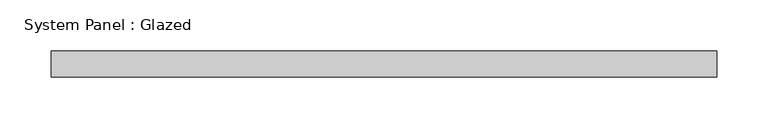
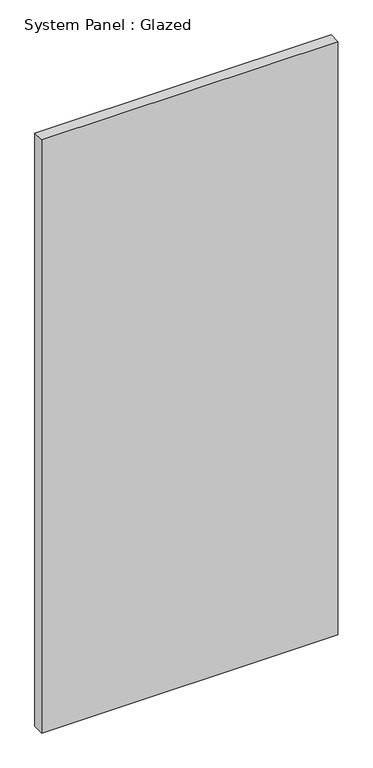
"""IFC4 building model written with IfcOpenShell, lengths in millimetres: plate geometry, System Panel : Glazed."""

from ifc_helpers import new_model, si_unit, origin, origin_with_axes, place, context, project, spatial, polyline, outline, extrude, source, transform, mapped, element, save


def system_panel_glazed_27f6d1d6(model_context):
    return source(origin(), model_context, "Body", "SweptSolid", [
        extrude(outline(polyline([(323.85, 19.05), (-323.85, 19.05), (-323.85, 44.45), (323.85, 44.45), (323.85, 19.05)])), origin_with_axes(), (0.0, 0.0, 1.0), 1371.695751),
    ])


if __name__ == "__main__":
    model = new_model("IFC4")
    model_context = context("Model", 3, world=origin())
    ifc_project = project(units=[si_unit("LENGTHUNIT", "METRE", prefix="MILLI")], contexts=[model_context])
    site = spatial("IfcSite", under=ifc_project)
    building = spatial("IfcBuilding", under=site)
    placement = place(None, origin())
    system_panel_glazed_shape = system_panel_glazed_27f6d1d6(model_context)
    element("IfcPlate", 1, ObjectType="System Panel : Glazed", at=placement, inside=building, context=model_context, shape_type="MappedRepresentation", body=[
        mapped(system_panel_glazed_shape, transform((0.0, 0.0, 0.0), x_axis=(1.0, 0.0, 0.0), y_axis=(0.0, 1.0, 0.0), z_axis=(0.0, 0.0, 1.0))),
    ])
    save(model, "model.ifc")

# Revit data of these elements
# Type "System Panel : Glazed"
#   Construction Type Id = "GSP4R"
#   Analytic Construction = "1/8 in Pilkington single glazing"
#   Visual Light Transmittance = 0.9
#   Solar Heat Gain Coefficient = 0.86
#   Heat Transfer Coefficient (U) = 1.18115 BTU/(h·ft²·°F)
#   Define Thermal Properties by = 1
# Element 1 (IfcPlate, "System Panel : Glazed")
#   Materials on its faces: "Glass"
# Materials
#   "Glass": class "Glass", colour RGB 0 128 192, transparency 0.75, Description = "Soda Lime Glass", Cost = 0
